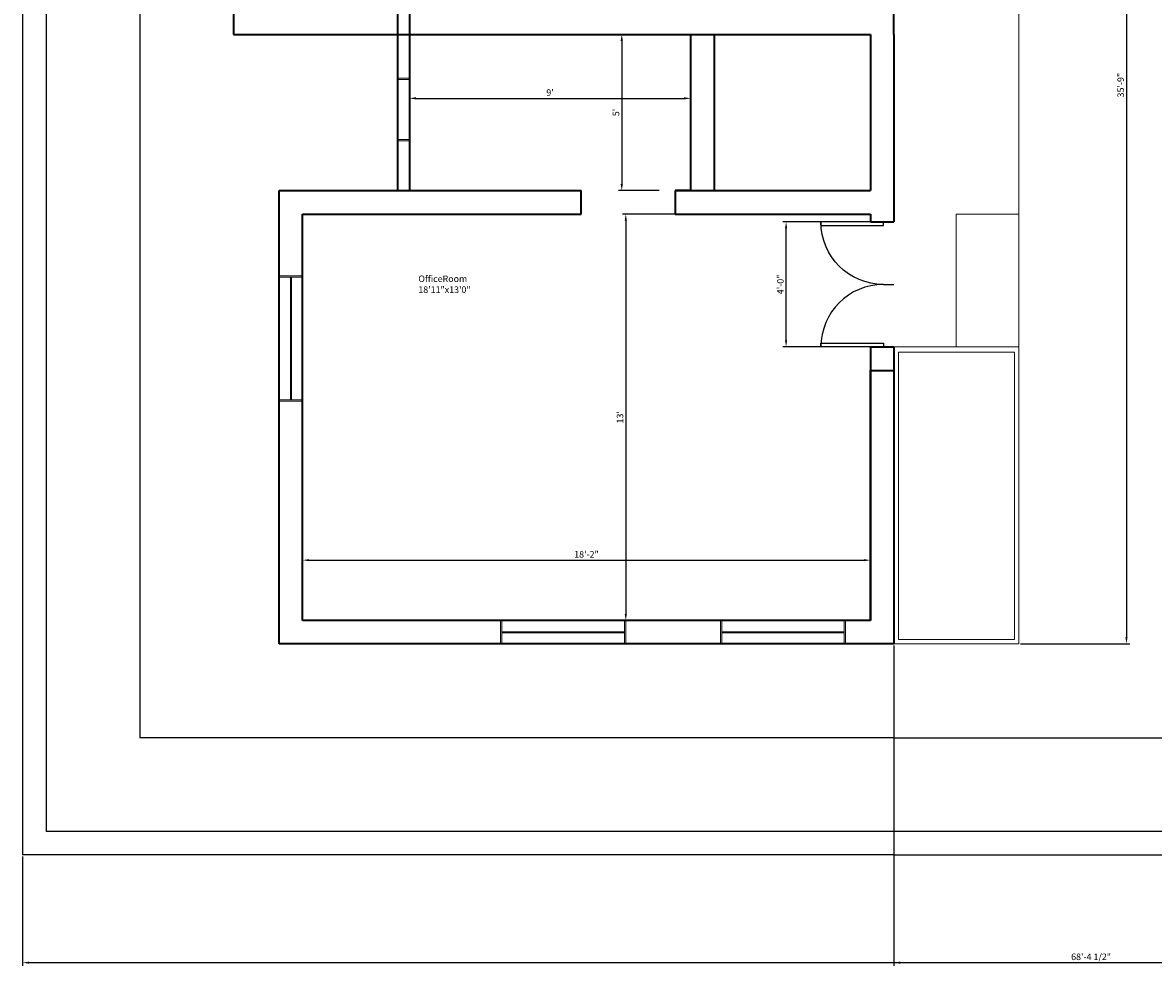
# Model space of a CAD drawing. Units: inches. Extents: x 250205121 to 250208111, y 89832590 to 89833271.
# Tile 1 of 14: x 250205166 to 250205601, y 89832590 to 89832953. Entities that reach past the tile are written whole.
import ezdxf

# ---------------------------------------------------------------- set-up
doc = ezdxf.new("R2010")
doc.units = ezdxf.units.IN
for name, color, linetype, lineweight in [('A-AREA-IDEN', 4, 'Continuous', 18), ('A-FLOR', 7, 'Continuous', 18), ('A-WALL', 7, 'Continuous', 35), ('C-PROP', 8, 'Continuous', 25), ('dimensions', 2, 'Continuous', 18), ('doors', 3, 'Continuous', 25), ('window', 4, 'Continuous', 18)]:
    doc.layers.add(name, color=color, linetype=linetype, lineweight=lineweight)
doc.styles.get("Standard").update_dxf_attribs({"font": 'arial.ttf'})
doc.dimstyles.new('ISO-25', dxfattribs={"dimtxt": 2.5, "dimasz": 2.5, "dimexe": 1.25, "dimexo": 0.625, "dimtad": 1, "dimlunit": 4, "dimtxsty": 'Standard', "dimcen": 2.5, "dimadec": 0, "dimazin": 0, "dimtfac": 1, "dimtmove": 0, "dimatfit": 3, "dimfxl": 1, "dimarcsym": 0})

# ---------------------------------------------------------------- blocks, each defined once
blk = doc.blocks.new('*U2')
for p, q in [((0, 0), (0, -5)), ((30, 0), (30, -5))]:
    blk.add_line(p, q)
blk.add_lwpolyline([(0, 0), (0, 30), (1.75, 30), (1.75, 0)], close=True)
blk.add_arc((0, 0), 30, 0, 90)
blk = doc.blocks.new('*D5')
at = {"layer": 'Defpoints', "color": 0, "transparency": 16777216}
for p in [(250205273.91, 89832776.02), (250205491.91, 89832771.33), (250205491.91, 89832746.49)]:
    blk.add_point(p, dxfattribs=at)
at = {"layer": 'dimensions', "color": 0, "lineweight": -2, "transparency": 16777216}
for p, q in [((250205273.91, 89832775.4), (250205273.91, 89832745.24)), ((250205491.91, 89832770.7), (250205491.91, 89832745.24)), ((250205276.41, 89832746.49), (250205489.41, 89832746.49))]:
    blk.add_line(p, q, dxfattribs=at)
at = {"layer": 'dimensions', "color": 0, "transparency": 16777216}
for points in [[(250205276.41, 89832746.9), (250205276.41, 89832746.07), (250205273.91, 89832746.49)], [(250205489.41, 89832746.9), (250205489.41, 89832746.07), (250205491.91, 89832746.49)]]:
    blk.add_solid(points, dxfattribs=at)
at = {"layer": 'dimensions', "color": 0, "transparency": 16777216, "insert": (250205382.91, 89832748.39), "char_height": 2.5, "attachment_point": 5}
blk.add_mtext('18\'-2"', dxfattribs=at)
blk = doc.blocks.new('*D6')
at = {"layer": 'Defpoints', "color": 0, "transparency": 16777216}
for p in [(250205439.77, 89832879.33), (250205398.01, 89832723.33), (250205434.32, 89832723.33)]:
    blk.add_point(p, dxfattribs=at)
at = {"layer": 'dimensions', "color": 0, "lineweight": -2, "transparency": 16777216}
for p, q in [((250205439.15, 89832879.33), (250205396.76, 89832879.33)), ((250205398.01, 89832876.83), (250205398.01, 89832725.83)), ((250205433.7, 89832723.33), (250205396.76, 89832723.33))]:
    blk.add_line(p, q, dxfattribs=at)
at = {"layer": 'dimensions', "color": 0, "transparency": 16777216}
for points in [[(250205397.6, 89832876.83), (250205398.43, 89832876.83), (250205398.01, 89832879.33)], [(250205397.6, 89832725.83), (250205398.43, 89832725.83), (250205398.01, 89832723.33)]]:
    blk.add_solid(points, dxfattribs=at)
at = {"layer": 'dimensions', "color": 0, "transparency": 16777216, "insert": (250205396.11, 89832801.33), "char_height": 2.5, "attachment_point": 5, "rotation": 90}
blk.add_mtext("13'", dxfattribs=at)
blk = doc.blocks.new('*D7')
at = {"layer": 'Defpoints', "color": 0, "transparency": 16777216}
for p in [(250205314.91, 89832936.19), (250205422.91, 89832936.19), (250205422.91, 89832923.76)]:
    blk.add_point(p, dxfattribs=at)
at = {"layer": 'dimensions', "color": 0, "lineweight": -2, "transparency": 16777216}
for p, q in [((250205314.91, 89832935.57), (250205314.91, 89832922.51)), ((250205422.91, 89832935.57), (250205422.91, 89832922.51)), ((250205317.41, 89832923.76), (250205420.41, 89832923.76))]:
    blk.add_line(p, q, dxfattribs=at)
at = {"layer": 'dimensions', "color": 0, "transparency": 16777216}
for points in [[(250205317.41, 89832924.18), (250205317.41, 89832923.35), (250205314.91, 89832923.76)], [(250205420.41, 89832924.18), (250205420.41, 89832923.35), (250205422.91, 89832923.76)]]:
    blk.add_solid(points, dxfattribs=at)
at = {"layer": 'dimensions', "color": 0, "transparency": 16777216, "insert": (250205368.91, 89832925.66), "char_height": 2.5, "attachment_point": 5}
blk.add_mtext("9'", dxfattribs=at)
blk = doc.blocks.new('*D8')
at = {"layer": 'Defpoints', "color": 0, "transparency": 16777216}
for p in [(250205412.66, 89832948.33), (250205396.47, 89832888.33), (250205411.49, 89832888.33)]:
    blk.add_point(p, dxfattribs=at)
at = {"layer": 'dimensions', "color": 0, "lineweight": -2, "transparency": 16777216}
for p, q in [((250205412.04, 89832948.33), (250205395.22, 89832948.33)), ((250205396.47, 89832945.83), (250205396.47, 89832890.83)), ((250205410.86, 89832888.33), (250205395.22, 89832888.33))]:
    blk.add_line(p, q, dxfattribs=at)
at = {"layer": 'dimensions', "color": 0, "transparency": 16777216}
for points in [[(250205396.05, 89832945.83), (250205396.89, 89832945.83), (250205396.47, 89832948.33)], [(250205396.05, 89832890.83), (250205396.89, 89832890.83), (250205396.47, 89832888.33)]]:
    blk.add_solid(points, dxfattribs=at)
at = {"layer": 'dimensions', "color": 0, "transparency": 16777216, "insert": (250205394.57, 89832918.33), "char_height": 2.5, "attachment_point": 5, "rotation": 90}
blk.add_mtext("5'", dxfattribs=at)
blk = doc.blocks.new('WIN-48IN')
for p, q in [((0, 0), (0, 48.08)), ((0, 48.08), (9, 48.08)), ((9, 48.08), (9, 0)), ((0, 47.58), (9, 47.58)), ((4.3, 47.58), (4.3, 0.5)), ((4.7, 47.58), (4.7, 0.5)), ((9, 0.5), (0, 0.5)), ((9, 0), (0, 0))]:
    blk.add_line(p, q)
blk = doc.blocks.new('*D41')
at = {"layer": 'Defpoints', "color": 0, "transparency": 16777216}
for p in [(250205166.41, 89832633.33), (250205986.91, 89832633.33), (250205986.91, 89832591.98)]:
    blk.add_point(p, dxfattribs=at)
at = {"layer": 'dimensions', "color": 0, "lineweight": -2, "transparency": 16777216}
for p, q in [((250205166.41, 89832632.7), (250205166.41, 89832590.73)), ((250205986.91, 89832632.7), (250205986.91, 89832590.73)), ((250205168.91, 89832591.98), (250205984.41, 89832591.98))]:
    blk.add_line(p, q, dxfattribs=at)
at = {"layer": 'dimensions', "color": 0, "transparency": 16777216}
for points in [[(250205168.91, 89832592.39), (250205168.91, 89832591.56), (250205166.41, 89832591.98)], [(250205984.41, 89832592.39), (250205984.41, 89832591.56), (250205986.91, 89832591.98)]]:
    blk.add_solid(points, dxfattribs=at)
at = {"layer": 'dimensions', "color": 0, "transparency": 16777216, "insert": (250205576.66, 89832593.9), "char_height": 2.5, "attachment_point": 5}
blk.add_mtext('68\'-4 1/2"', dxfattribs=at)
blk = doc.blocks.new('*D47')
at = {"layer": 'Defpoints', "color": 0, "transparency": 16777216}
for p in [(250205500.91, 89832714.33), (250205797.91, 89832714.33), (250205797.91, 89832591.98)]:
    blk.add_point(p, dxfattribs=at)
at = {"layer": 'dimensions', "color": 0, "lineweight": -2, "transparency": 16777216}
for p, q in [((250205500.91, 89832713.7), (250205500.91, 89832590.73)), ((250205797.91, 89832713.7), (250205797.91, 89832590.73)), ((250205503.41, 89832591.98), (250205795.41, 89832591.98))]:
    blk.add_line(p, q, dxfattribs=at)
at = {"layer": 'dimensions', "color": 0, "transparency": 16777216}
for points in [[(250205503.41, 89832592.39), (250205503.41, 89832591.56), (250205500.91, 89832591.98)], [(250205795.41, 89832592.39), (250205795.41, 89832591.56), (250205797.91, 89832591.98)]]:
    blk.add_solid(points, dxfattribs=at)
at = {"layer": 'dimensions', "color": 0, "transparency": 16777216, "insert": (250205649.41, 89832593.88), "char_height": 2.5, "attachment_point": 5}
blk.add_mtext('24\'-9"', dxfattribs=at)
blk = doc.blocks.new('*D48')
at = {"layer": 'Defpoints', "color": 0, "transparency": 16777216}
for p in [(250205548.91, 89833143.33), (250205548.91, 89832714.33), (250205590.26, 89832714.33)]:
    blk.add_point(p, dxfattribs=at)
at = {"layer": 'dimensions', "color": 0, "lineweight": -2, "transparency": 16777216}
for p, q in [((250205549.53, 89833143.33), (250205591.51, 89833143.33)), ((250205590.26, 89833140.83), (250205590.26, 89832716.83)), ((250205549.53, 89832714.33), (250205591.51, 89832714.33))]:
    blk.add_line(p, q, dxfattribs=at)
at = {"layer": 'dimensions', "color": 0, "transparency": 16777216}
for points in [[(250205589.84, 89833140.83), (250205590.67, 89833140.83), (250205590.26, 89833143.33)], [(250205589.84, 89832716.83), (250205590.67, 89832716.83), (250205590.26, 89832714.33)]]:
    blk.add_solid(points, dxfattribs=at)
at = {"layer": 'dimensions', "color": 0, "transparency": 16777216, "insert": (250205588.36, 89832928.83), "char_height": 2.5, "attachment_point": 5, "rotation": 90}
blk.add_mtext('35\'-9"', dxfattribs=at)
blk = doc.blocks.new('*D52')
at = {"layer": 'Defpoints', "color": 0, "transparency": 16777216}
for p in [(250205459.56, 89832876.33), (250205500.91, 89832876.33), (250205500.91, 89832828.33)]:
    blk.add_point(p, dxfattribs=at)
at = {"layer": 'dimensions', "color": 0, "lineweight": -2, "transparency": 16777216}
for p, q in [((250205500.28, 89832876.33), (250205458.31, 89832876.33)), ((250205459.56, 89832830.83), (250205459.56, 89832873.83)), ((250205500.28, 89832828.33), (250205458.31, 89832828.33))]:
    blk.add_line(p, q, dxfattribs=at)
at = {"layer": 'dimensions', "color": 0, "transparency": 16777216}
for points in [[(250205459.14, 89832873.83), (250205459.97, 89832873.83), (250205459.56, 89832876.33)], [(250205459.14, 89832830.83), (250205459.97, 89832830.83), (250205459.56, 89832828.33)]]:
    blk.add_solid(points, dxfattribs=at)
at = {"layer": 'dimensions', "color": 0, "transparency": 16777216, "insert": (250205457.66, 89832852.33), "char_height": 2.5, "attachment_point": 5, "rotation": 90}
blk.add_mtext('4\'-0"', dxfattribs=at)

msp = doc.modelspace()

# ---------------------------------------------------------------- linework, layer by layer
at = {"layer": 'A-FLOR'}
for p, q in [((250205548.908, 89833143.328), (250205548.908, 89832714.328)), ((250205524.908, 89832828.328), (250205524.908, 89832879.328)), ((250205524.908, 89832879.328), (250205548.908, 89832879.328)), ((250205500.908, 89832828.328), (250205548.908, 89832828.328)), ((250205548.908, 89832714.328), (250205500.908, 89832714.328))]:
    msp.add_line(p, q, dxfattribs=at)
msp.add_lwpolyline([(250205502.76, 89832826.329), (250205547.227, 89832826.329), (250205547.227, 89832716.018), (250205502.76, 89832716.018)], close=True, dxfattribs=at)
at = {"layer": 'A-WALL'}
for p, q in [((250205500.908, 89832948.328), (250205500.908, 89833134.328)), ((250205314.908, 89833045.828), (250205314.908, 89832888.328)), ((250205310.408, 89833041.328), (250205310.408, 89832888.328)), ((250205247.408, 89832999.328), (250205247.408, 89832948.328)), ((250205247.408, 89832948.328), (250205491.908, 89832948.328)), ((250205422.908, 89832948.328), (250205422.908, 89832888.328)), ((250205431.908, 89832948.328), (250205431.908, 89832888.328)), ((250205491.908, 89832948.328), (250205491.908, 89832888.328)), ((250205500.908, 89832948.328), (250205500.908, 89832879.328)), ((250205264.908, 89832888.328), (250205380.908, 89832888.328)), ((250205264.908, 89832714.328), (250205264.908, 89832888.328)), ((250205380.908, 89832879.328), (250205380.908, 89832888.328)), ((250205422.908, 89832888.328), (250205416.908, 89832888.328)), ((250205416.908, 89832888.328), (250205416.908, 89832879.328)), ((250205416.908, 89832888.328), (250205491.908, 89832888.328)), ((250205273.908, 89832879.328), (250205380.908, 89832879.328)), ((250205273.908, 89832723.328), (250205273.908, 89832879.328)), ((250205416.908, 89832879.328), (250205491.908, 89832879.328)), ((250205491.908, 89832879.328), (250205491.908, 89832876.328)), ((250205500.908, 89832879.328), (250205500.908, 89832876.328)), ((250205491.908, 89832876.328), (250205500.908, 89832876.328)), ((250205491.908, 89832828.328), (250205500.908, 89832828.328)), ((250205491.908, 89832828.328), (250205491.908, 89832723.328)), ((250205500.908, 89832828.328), (250205500.908, 89832723.328)), ((250205491.908, 89832801.328), (250205491.908, 89832819.328)), ((250205491.908, 89832819.328), (250205500.908, 89832819.328)), ((250205491.908, 89832741.328), (250205491.908, 89832801.328)), ((250205491.908, 89832723.328), (250205491.908, 89832741.328)), ((250205491.908, 89832723.328), (250205273.908, 89832723.328)), ((250205500.908, 89832723.328), (250205500.908, 89832714.328)), ((250205273.908, 89832714.328), (250205264.908, 89832714.328)), ((250205500.908, 89832714.328), (250205273.908, 89832714.328))]:
    msp.add_line(p, q, dxfattribs=at)
at = {"layer": 'C-PROP'}
for p, q in [((250205166.408, 89833224.328), (250205166.408, 89832633.328)), ((250205175.408, 89833215.328), (250205175.408, 89832642.328)), ((250205211.408, 89833179.328), (250205211.408, 89832678.328)), ((250205500.908, 89832678.328), (250205211.408, 89832678.328)), ((250205500.908, 89832678.328), (250205941.908, 89832678.328)), ((250205500.908, 89832642.328), (250205175.408, 89832642.328)), ((250205977.908, 89832642.328), (250205500.908, 89832642.328)), ((250205500.908, 89832633.328), (250205166.408, 89832633.328)), ((250205500.908, 89832633.328), (250205977.908, 89832633.328))]:
    msp.add_line(p, q, dxfattribs=at)
at = {"layer": 'window'}
for p, q in [((250205310.408, 89832931.515), (250205314.908, 89832931.515)), ((250205310.408, 89832931.015), (250205314.908, 89832931.015)), ((250205310.608, 89832931.015), (250205310.608, 89832907.936)), ((250205314.908, 89832931.515), (250205314.908, 89832907.436)), ((250205314.908, 89832907.936), (250205310.408, 89832907.936)), ((250205314.908, 89832907.436), (250205310.408, 89832907.436))]:
    msp.add_line(p, q, dxfattribs=at)

# ---------------------------------------------------------------- block references
at = {"layer": 'doors', "yscale": 0.8, "zscale": 0.8, "rotation": 90}
for p, xscale in [((250205496.908, 89832876.328), -0.8), ((250205496.908, 89832828.328), 0.8)]:
    msp.add_blockref('*U2', p, dxfattribs=dict(at, xscale=xscale))
at = {"layer": 'window'}
msp.add_blockref('WIN-48IN', (250205264.908, 89832807.501), dxfattribs=at)
for p, rotation in [((250205398.013, 89832714.328), 90.00000001284631), ((250205482.403, 89832714.328), 89.99999996146099)]:
    msp.add_blockref('WIN-48IN', p, dxfattribs=dict(at, rotation=rotation))

# ---------------------------------------------------------------- texts
at = {"layer": 'A-AREA-IDEN', "insert": (250205318.354, 89832855.748), "char_height": 2.5, "attachment_point": 1}
msp.add_mtext_dynamic_manual_height_columns('OfficeRoom\\P18\'11"x13\'0"', width=2.73747, gutter_width=12.5, heights=[0], dxfattribs=at)

# ---------------------------------------------------------------- dimensions: what is measured, and where the dimension line sits
at = {"layer": 'dimensions'}
for base, p1, p2, angle, override, picture, middle in [((250205590.258, 89832714.328), (250205548.908, 89833143.328), (250205548.908, 89832714.328), 270, {"dimdec": 1, "dimlfac": 1, "dimrnd": 0, "dimzin": 1, "dimdsep": 46, "dimlunit": 4, "dimfrac": 2}, '*D48', (250205588.355, 89832928.828)), ((250205396.469, 89832888.328), (250205412.661, 89832948.328), (250205411.488, 89832888.328), 90, {"dimclrd": 0, "dimclre": 0, "dimclrt": 0}, '*D8', (250205394.573, 89832918.328)), ((250205398.013, 89832723.328), (250205439.772, 89832879.328), (250205434.324, 89832723.328), 90, {"dimclrd": 0, "dimclre": 0, "dimclrt": 0}, '*D6', (250205396.111, 89832801.328)), ((250205459.558, 89832876.328), (250205500.908, 89832828.328), (250205500.908, 89832876.328), 90, {"dimdec": 1, "dimlfac": 1, "dimrnd": 0, "dimzin": 1, "dimdsep": 46, "dimlunit": 4, "dimfrac": 2}, '*D52', (250205457.656, 89832852.328))]:
    dim = msp.add_linear_dim(base=base, p1=p1, p2=p2, angle=angle, dimstyle='ISO-25', override=override, dxfattribs=at)
    dim.commit()
    dim.dimension.update_dxf_attribs({"geometry": picture, "text_midpoint": middle})
for base, p1, p2, override, picture, middle in [((250205422.908, 89832923.762), (250205314.908, 89832936.19), (250205422.908, 89832936.19), {"dimclrd": 0, "dimclre": 0, "dimclrt": 0}, '*D7', (250205368.908, 89832925.663)), ((250205491.908, 89832746.487), (250205273.908, 89832776.021), (250205491.908, 89832771.328), {"dimclrd": 0, "dimclre": 0, "dimclrt": 0}, '*D5', (250205382.908, 89832748.388)), ((250205797.908, 89832591.978), (250205500.908, 89832714.328), (250205797.908, 89832714.328), {"dimdec": 1, "dimlfac": 1, "dimrnd": 0, "dimzin": 1, "dimdsep": 46, "dimlunit": 4, "dimfrac": 2}, '*D47', (250205649.408, 89832593.879)), ((250205986.908, 89832591.978), (250205166.408, 89832633.328), (250205986.908, 89832633.328), {"dimdec": 1, "dimlfac": 1, "dimrnd": 0, "dimzin": 1, "dimdsep": 46, "dimlunit": 4, "dimfrac": 2}, '*D41', (250205576.658, 89832593.896))]:
    dim = msp.add_linear_dim(base=base, p1=p1, p2=p2, dimstyle='ISO-25', override=override, dxfattribs=at)
    dim.commit()
    dim.dimension.update_dxf_attribs({"geometry": picture, "text_midpoint": middle})

doc.saveas('drawing.dxf')
